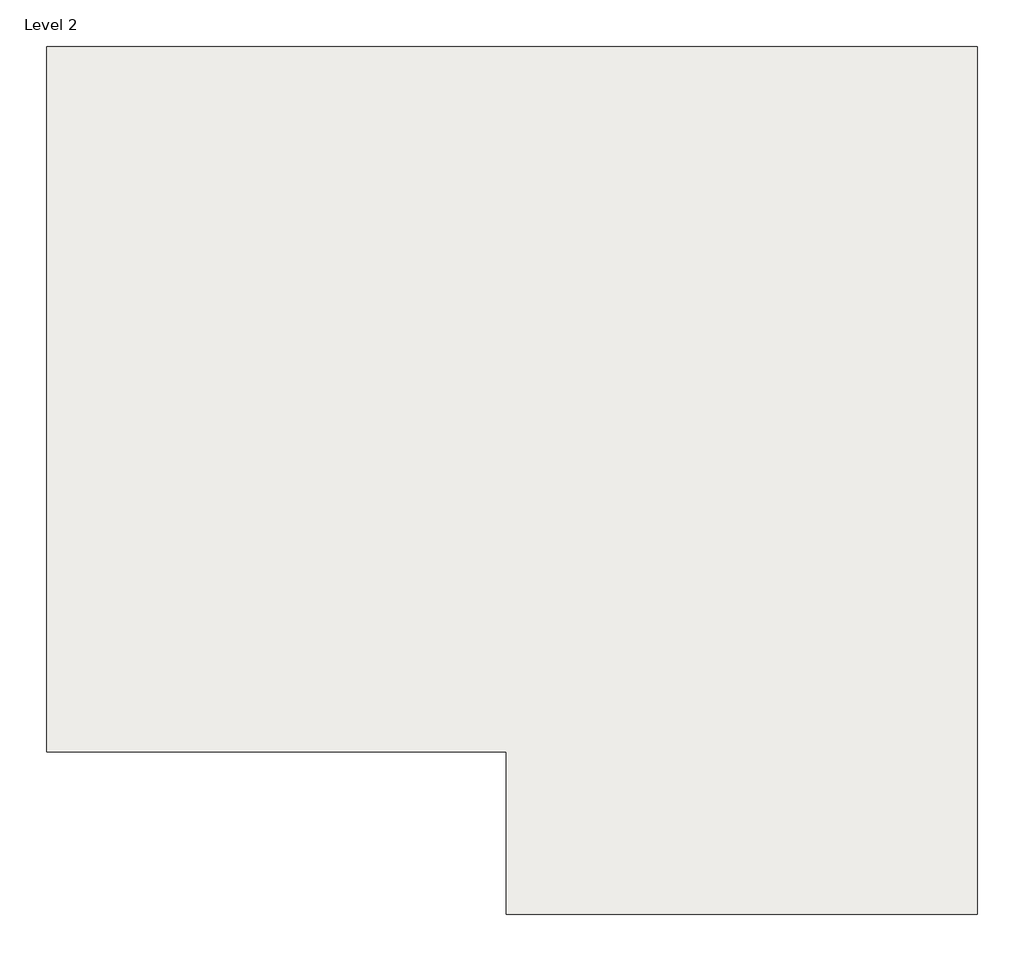
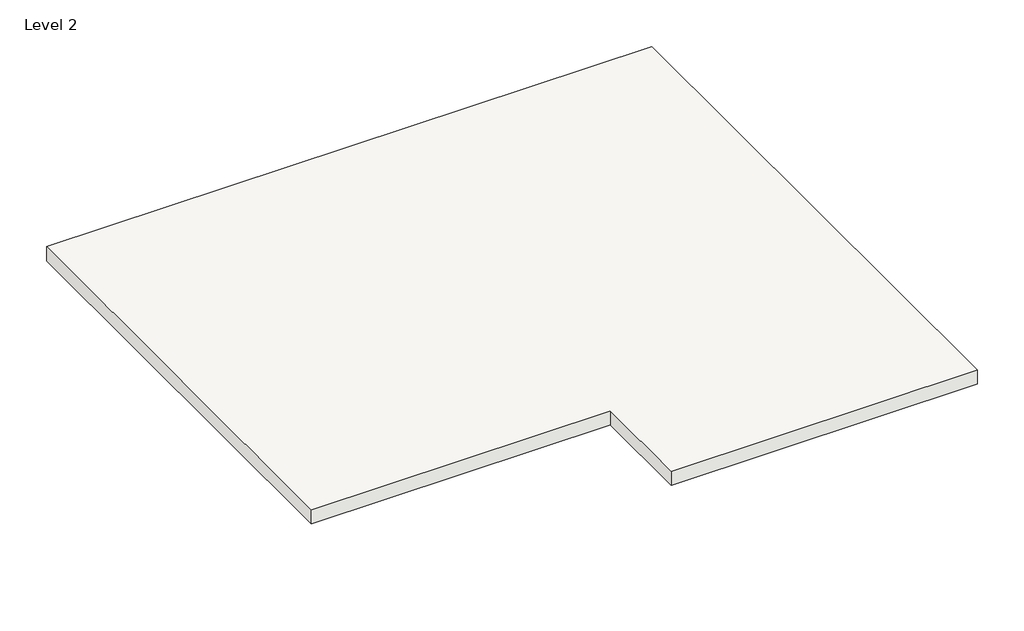
# One storey: 1 roof.
"""IFC4 building model written with IfcOpenShell, lengths in millimetres."""

from ifc_helpers import new_model, si_unit, frame, origin, place, context, project, spatial, polyline, outline, extrude, element, save

model = new_model("IFC4")

# Units and contexts
model_context = context("Model", 3, world=origin())
ifc_project = project(units=[si_unit("LENGTHUNIT", "METRE", prefix="MILLI")], contexts=[model_context])

# Site, building, storey
site = spatial("IfcSite", under=ifc_project)
building = spatial("IfcBuilding", under=site)
storey = spatial("IfcBuildingStorey", under=building, Name="Level 2", Elevation=3048.0)

# Roof
placement = place(None, origin())
element("IfcRoof", 1, ObjectType="Generic - 12\"", at=placement, inside=storey, context=model_context, shape_type="SweptSolid", body=[
    extrude(outline(polyline([(-5152.4621755, 8759.7807133), (7242.7378245, 8759.7807133), (7242.7378245, -2797.2192867), (968.9378245, -2797.2192867), (968.9378245, -638.2192867), (-5152.4621755, -638.2192867), (-5152.4621755, 8759.7807133)])), frame((0.0, 0.0, 3048.0), z_axis=(0.0, 0.0, 1.0), x_axis=(1.0, 0.0, 0.0)), (0.0, 0.0, 1.0), 304.8),
])

save(model, "model.ifc")

# Revit data of these elements
# Type "Generic - 12\""
#   Assembly Code = "B1020"
#   Layers, outside or top first: 1' - 0" "Brick, Soldier Course" (function 1)
# Element 1 (IfcRoof, "Generic - 12\"")
#   built-in parameter 1001705 = 11 (stored number, unit not read)
#   built-in parameter 1001710 = 33615
#   Phase Created = New Construction
#   Materials on its faces: "Brick, Soldier Course"
# Materials
#   "Brick, Soldier Course": class "Masonry", colour RGB 170 98 104, transparency 0, Description = "Common brick soldier coursed", Cost = 0
